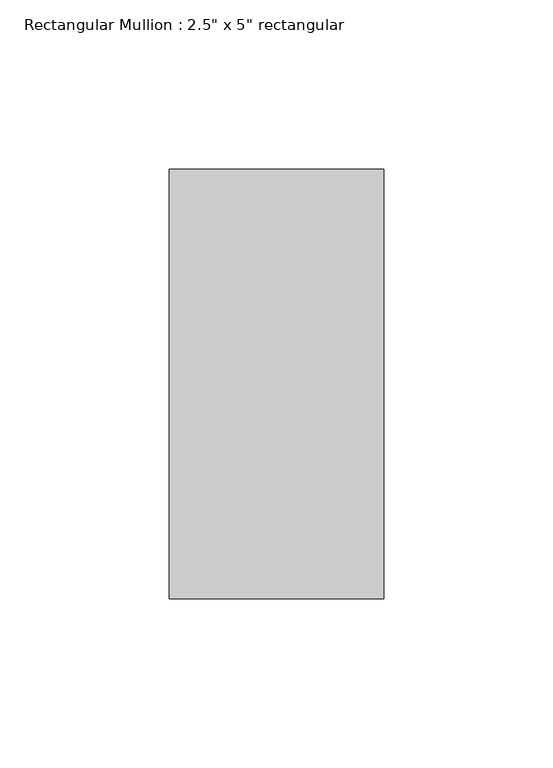
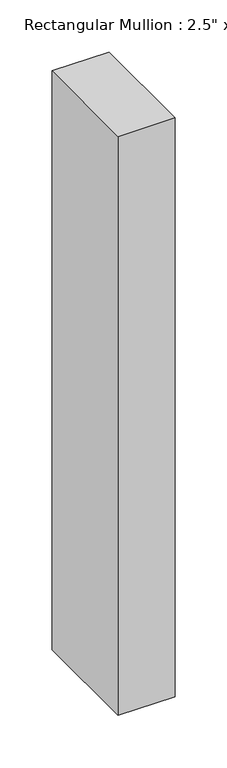
"""IFC4 building model written with IfcOpenShell, lengths in millimetres: member geometry."""

from ifc_helpers import new_model, si_unit, frame, origin, place, context, project, spatial, polyline, outline, extrude, source, transform, mapped, element, save


def member_8613ee48(model_context):
    return source(origin(), model_context, "Body", "SweptSolid", [
        extrude(outline(polyline([(0.0, 63.5), (0.0, -63.5), (-63.5, -63.5), (-63.5, 63.5), (0.0, 63.5)])), frame((0.0, 0.0, -679.45), z_axis=(0.0, 0.0, 1.0), x_axis=(1.0, 0.0, 0.0)), (0.0, 0.0, 1.0), 679.45),
    ])


if __name__ == "__main__":
    model = new_model("IFC4")
    model_context = context("Model", 3, world=origin())
    ifc_project = project(units=[si_unit("LENGTHUNIT", "METRE", prefix="MILLI")], contexts=[model_context])
    site = spatial("IfcSite", under=ifc_project)
    building = spatial("IfcBuilding", under=site)
    placement = place(None, origin())
    member_shape = member_8613ee48(model_context)
    element("IfcMember", 1, ObjectType="Rectangular Mullion : 2.5\" x 5\" rectangular", at=placement, inside=building, context=model_context, shape_type="MappedRepresentation", body=[
        mapped(member_shape, transform((0.0, 0.0, 0.0), x_axis=(1.0, 0.0, 0.0), y_axis=(0.0, 1.0, 0.0), z_axis=(0.0, 0.0, 1.0))),
    ])
    save(model, "model.ifc")

# Revit data of these elements
# Type "Rectangular Mullion : 2.5\" x 5\" rectangular"
#   built-in parameter 1007304 = 0.416667 (stored number, unit not read)
#   built-in parameter 1007301 = 0.104167 (stored number, unit not read)
#   built-in parameter 1007300 = 0.104167 (stored number, unit not read)
# Element 1 (IfcMember, "Rectangular Mullion : 2.5\" x 5\" rectangular")
#   Materials on its faces: "Aluminum"
# Materials
#   "Aluminum": class "Metal", colour RGB 247 247 247, transparency 0, Description = "Aluminum 6061", Cost = 0
